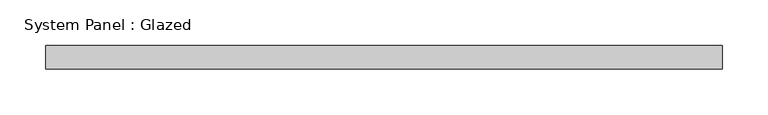
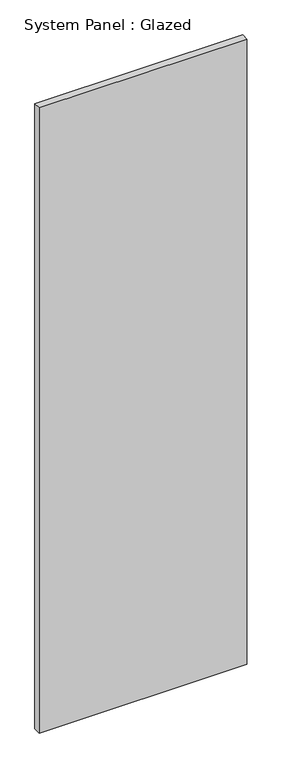
"""IFC4 building model written with IfcOpenShell, lengths in millimetres: plate geometry, System Panel : Glazed."""

from ifc_helpers import new_model, si_unit, origin, origin_with_axes, place, context, project, spatial, polyline, outline, extrude, source, transform, mapped, element, save


def system_panel_glazed_091cc013(model_context):
    return source(origin(), model_context, "Body", "SweptSolid", [
        extrude(outline(polyline([(368.3, 19.05), (-368.3, 19.05), (-368.3, 44.45), (368.3, 44.45), (368.3, 19.05)])), origin_with_axes(), (0.0, 0.0, 1.0), 2343.15),
    ])


if __name__ == "__main__":
    model = new_model("IFC4")
    model_context = context("Model", 3, world=origin())
    ifc_project = project(units=[si_unit("LENGTHUNIT", "METRE", prefix="MILLI")], contexts=[model_context])
    site = spatial("IfcSite", under=ifc_project)
    building = spatial("IfcBuilding", under=site)
    placement = place(None, origin())
    system_panel_glazed_shape = system_panel_glazed_091cc013(model_context)
    element("IfcPlate", 1, ObjectType="System Panel : Glazed", at=placement, inside=building, context=model_context, shape_type="MappedRepresentation", body=[
        mapped(system_panel_glazed_shape, transform((0.0, 0.0, 0.0), x_axis=(1.0, 0.0, 0.0), y_axis=(0.0, 1.0, 0.0), z_axis=(0.0, 0.0, 1.0))),
    ])
    save(model, "model.ifc")

# Revit data of these elements
# Type "System Panel : Glazed"
#   Construction Type Id = "GSP4R"
#   Analytic Construction = "1/8 in Pilkington single glazing"
#   Visual Light Transmittance = 0.9
#   Solar Heat Gain Coefficient = 0.86
#   Heat Transfer Coefficient (U) = 1.18115 BTU/(h·ft²·°F)
#   Define Thermal Properties by = 1
# Element 1 (IfcPlate, "System Panel : Glazed")
#   Materials on its faces: "Glass"
# Materials
#   "Glass": class "Glass", colour RGB 0 128 192, transparency 0.75, Description = "Soda Lime Glass", Cost = 0
